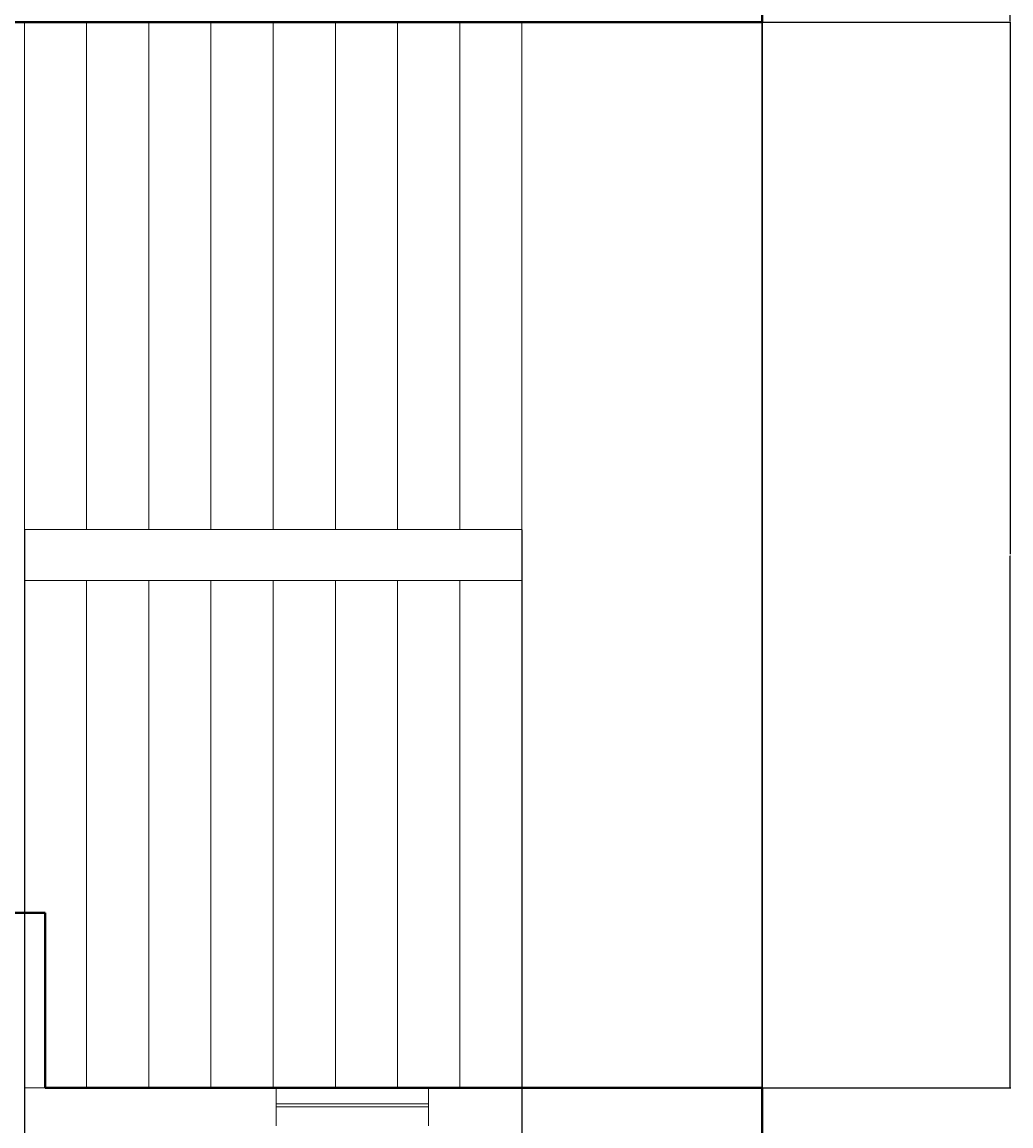
# Model space of a CAD drawing. Units: inches. Extents: x -46 to 1145, y -527 to 760.
# Tile 22 of 57: x 912 to 1145, y -39 to 222. Entities that reach past the tile are written whole.
import ezdxf

# ---------------------------------------------------------------- set-up
doc = ezdxf.new("R2010")
doc.units = ezdxf.units.IN
doc.header["$MEASUREMENT"] = 0
for name, color, linetype, lineweight in [('A-ANNO-DIMS', 2, 'Continuous', 18), ('A-FLOR-STRS', 5, 'Continuous', 20), ('C-SITE', 7, 'Continuous', 30), ('WALLS', 4, 'Continuous', 40), ('WINDOWS', 240, 'Continuous', 20)]:
    doc.layers.add(name, color=color, linetype=linetype, lineweight=lineweight)
doc.styles.get("Standard").update_dxf_attribs({"font": 'arial.ttf'})
doc.dimstyles.get("Standard").update_dxf_attribs({"dimtxt": 0.18, "dimasz": 0.18, "dimexe": 0.18, "dimexo": 0.0625, "dimgap": 0.09, "dimtad": 0, "dimtih": 1, "dimtoh": 1, "dimdec": 0, "dimzin": 0, "dimdsep": 46, "dimlunit": 3, "dimtxsty": 'Standard', "dimcen": 0.09, "dimadec": 0, "dimazin": 0, "dimtfac": 1, "dimtdec": 0, "dimtofl": 0, "dimtmove": 0, "dimatfit": 3, "dimfxl": 1, "dimtolj": 1, "dimtzin": 0, "dimarcsym": 0})

# ---------------------------------------------------------------- blocks, each defined once
blk = doc.blocks.new('WINDOW-36IN')
for p, q in [((0, 4.5), (0, 9)), ((0, 9), (0, 0)), ((36, 9), (36, 0)), ((0, 5.23), (36, 5.23)), ((0, 4.5), (36, 4.5))]:
    blk.add_line(p, q)
blk = doc.blocks.new('*D688')
at = {"layer": 'A-ANNO-DIMS', "color": 0, "lineweight": -2, "transparency": 16777216}
for p, q in [((1086.63, 659.52), (1145.34, 659.52)), ((1145.16, 659.34), (1145.16, 440.7)), ((1145.16, 221.7), (1145.16, 440.34)), ((1086.63, 221.52), (1145.34, 221.52))]:
    blk.add_line(p, q, dxfattribs=at)
at = {"layer": 'A-ANNO-DIMS', "color": 0, "transparency": 16777216}
for points in [[(1145.13, 659.34), (1145.19, 659.34), (1145.16, 659.52)], [(1145.13, 221.7), (1145.19, 221.7), (1145.16, 221.52)]]:
    blk.add_solid(points, dxfattribs=at)
at = {"layer": 'Defpoints', "color": 0, "transparency": 16777216}
for p in [(1086.56, 659.52), (1145.16, 659.52), (1086.56, 221.52)]:
    blk.add_point(p, dxfattribs=at)
at = {"layer": 'A-ANNO-DIMS', "color": 0, "transparency": 16777216, "insert": (1145.16, 440.52), "char_height": 0.18, "attachment_point": 5}
blk.add_mtext('\\A1;438', dxfattribs=at)
blk = doc.blocks.new('*D689')
at = {"layer": 'A-ANNO-DIMS', "color": 0, "lineweight": -2, "transparency": 16777216}
for p, q in [((1086.63, 221.52), (1145.34, 221.52)), ((1145.16, 221.34), (1145.16, 95.7)), ((1145.16, -30.3), (1145.16, 95.34)), ((1086.63, -30.48), (1145.34, -30.48))]:
    blk.add_line(p, q, dxfattribs=at)
at = {"layer": 'A-ANNO-DIMS', "color": 0, "transparency": 16777216}
for points in [[(1145.13, 221.34), (1145.19, 221.34), (1145.16, 221.52)], [(1145.13, -30.3), (1145.19, -30.3), (1145.16, -30.48)]]:
    blk.add_solid(points, dxfattribs=at)
at = {"layer": 'Defpoints', "color": 0, "transparency": 16777216}
for p in [(1086.56, 221.52), (1145.16, 221.52), (1086.56, -30.48)]:
    blk.add_point(p, dxfattribs=at)
at = {"layer": 'A-ANNO-DIMS', "color": 0, "transparency": 16777216, "insert": (1145.16, 95.52), "char_height": 0.18, "attachment_point": 5}
blk.add_mtext('\\A1;252', dxfattribs=at)
blk = doc.blocks.new('*D694')
at = {"layer": 'A-ANNO-DIMS', "color": 0, "lineweight": -2, "transparency": 16777216}
for p, q in [((912.18, 101.46), (912.18, -527.26)), ((1029.77, 101.46), (1029.77, -527.26)), ((912.36, -527.08), (970.59, -527.08)), ((1029.59, -527.08), (971.36, -527.08))]:
    blk.add_line(p, q, dxfattribs=at)
at = {"layer": 'A-ANNO-DIMS', "color": 0, "transparency": 16777216}
for points in [[(912.36, -527.05), (912.36, -527.11), (912.18, -527.08)], [(1029.59, -527.05), (1029.59, -527.11), (1029.77, -527.08)]]:
    blk.add_solid(points, dxfattribs=at)
at = {"layer": 'Defpoints', "color": 0, "transparency": 16777216}
for p in [(912.18, 101.52), (1029.77, 101.52), (1029.77, -527.08)]:
    blk.add_point(p, dxfattribs=at)
at = {"layer": 'A-ANNO-DIMS', "color": 0, "transparency": 16777216, "insert": (970.97, -527.08), "char_height": 0.18, "attachment_point": 5}
blk.add_mtext('\\A1;117.6', dxfattribs=at)

msp = doc.modelspace()

# ---------------------------------------------------------------- linework, layer by layer
at = {"layer": 'A-FLOR-STRS'}
for p, q in [((912.1762, 221.5176), (912.1762, 101.5176)), ((926.8756, 221.5176), (926.8756, 101.5176)), ((941.575, 221.5176), (941.575, 101.5176)), ((956.2744, 221.5176), (956.2744, 101.5176)), ((970.9738, 221.5176), (970.9738, 101.5176)), ((985.6732, 221.5176), (985.6732, 101.5176)), ((1000.3726, 221.5176), (1000.3726, 101.5176)), ((1015.072, 221.5176), (1015.072, 101.5176)), ((1029.7714, 221.5176), (1029.7714, 101.5176)), ((1029.7714, 101.5176), (912.1762, 101.5176)), ((912.1762, 101.5176), (912.1762, -30.4824)), ((1029.7714, 101.5176), (1029.7714, -30.4824)), ((1029.7714, 89.5176), (912.1762, 89.5176)), ((926.8756, 89.5176), (926.8756, -30.4824)), ((941.575, 89.5176), (941.575, -30.4824)), ((956.2744, 89.5176), (956.2744, -30.4824)), ((970.9738, 89.5176), (970.9738, -30.4824)), ((985.6732, 89.5176), (985.6732, -30.4824)), ((1000.3726, 89.5176), (1000.3726, -30.4824)), ((1015.072, 89.5176), (1015.072, -30.4824)), ((912.1762, -30.4824), (1029.7714, -30.4824))]:
    msp.add_line(p, q, dxfattribs=at)
at = {"layer": 'C-SITE'}
msp.add_line((1086.5637, 221.5176), (1086.5637, -30.4824), dxfattribs=at)
at = {"layer": 'WALLS'}
for p, q in [((1086.5637, 221.5176), (1086.5637, 659.5176)), ((1086.5637, 221.5176), (821.7731, 221.5176)), ((767.0637, 10.8886), (917.0637, 10.8886)), ((917.0637, -30.4824), (917.0637, 10.8886)), ((917.0637, -30.4824), (1086.5637, -30.4824)), ((1086.5637, -30.4824), (1086.5637, -468.4824))]:
    msp.add_line(p, q, dxfattribs=at)

# ---------------------------------------------------------------- block references
at = {"layer": 'WINDOWS'}
msp.add_blockref('WINDOW-36IN', (971.6543, -39.482), dxfattribs=at)

# ---------------------------------------------------------------- dimensions: what is measured, and where the dimension line sits
at = {"layer": 'A-ANNO-DIMS'}
for base, p1, p2, picture, middle in [((1145.1637, 659.5176), (1086.5637, 221.5176), (1086.5637, 659.5176), '*D688', (1145.1637, 440.5176)), ((1145.1637, 221.5176), (1086.5637, -30.4824), (1086.5637, 221.5176), '*D689', (1145.1637, 95.5176))]:
    dim = msp.add_linear_dim(base=base, p1=p1, p2=p2, angle=90, dimstyle='Standard', override={"dimdec": 0, "dimlfac": 1, "dimrnd": 0, "dimzin": 0, "dimdsep": 46, "dimlunit": 2}, dxfattribs=at)
    dim.commit()
    dim.dimension.update_dxf_attribs({"geometry": picture, "text_midpoint": middle})
dim = msp.add_linear_dim(base=(1029.7714, -527.0824), p1=(912.1762, 101.5176), p2=(1029.7714, 101.5176), dimstyle='Standard', override={"dimdec": 1, "dimlfac": 1, "dimrnd": 0, "dimzin": 0, "dimdsep": 46, "dimlunit": 2}, dxfattribs=at)
dim.commit()
dim.dimension.update_dxf_attribs({"geometry": '*D694', "text_midpoint": (970.9738, -527.0824)})

doc.saveas('drawing.dxf')
